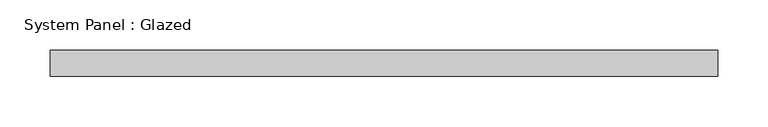
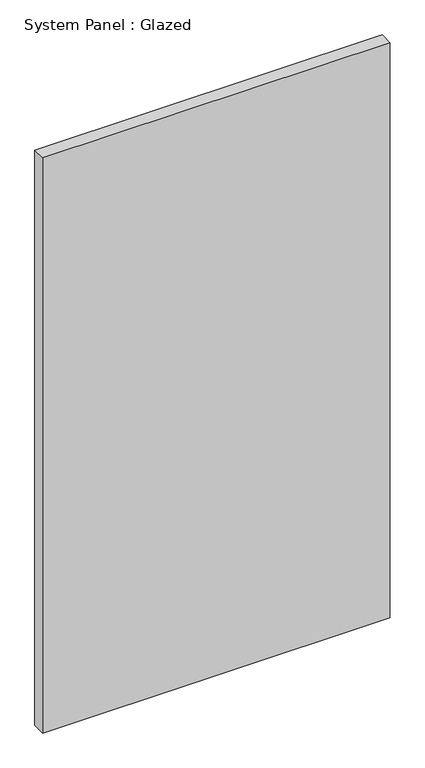
"""IFC4 building model written with IfcOpenShell, lengths in millimetres: plate geometry, System Panel : Glazed."""

from ifc_helpers import new_model, si_unit, origin, origin_with_axes, place, context, project, spatial, polyline, outline, extrude, source, transform, mapped, element, save


def system_panel_glazed_73c284ea(model_context):
    return source(origin(), model_context, "Body", "SweptSolid", [
        extrude(outline(polyline([(330.2, 19.05), (-330.2, 19.05), (-330.2, 44.45), (330.2, 44.45), (330.2, 19.05)])), origin_with_axes(), (0.0, 0.0, 1.0), 1155.7),
    ])


if __name__ == "__main__":
    model = new_model("IFC4")
    model_context = context("Model", 3, world=origin())
    ifc_project = project(units=[si_unit("LENGTHUNIT", "METRE", prefix="MILLI")], contexts=[model_context])
    site = spatial("IfcSite", under=ifc_project)
    building = spatial("IfcBuilding", under=site)
    placement = place(None, origin())
    system_panel_glazed_shape = system_panel_glazed_73c284ea(model_context)
    element("IfcPlate", 1, ObjectType="System Panel : Glazed", at=placement, inside=building, context=model_context, shape_type="MappedRepresentation", body=[
        mapped(system_panel_glazed_shape, transform((0.0, 0.0, 0.0), x_axis=(1.0, 0.0, 0.0), y_axis=(0.0, 1.0, 0.0), z_axis=(0.0, 0.0, 1.0))),
    ])
    save(model, "model.ifc")

# Revit data of these elements
# Type "System Panel : Glazed"
#   Construction Type Id = "GSP4R"
#   Analytic Construction = "1/8 in Pilkington single glazing"
#   Visual Light Transmittance = 0.9
#   Solar Heat Gain Coefficient = 0.86
#   Heat Transfer Coefficient (U) = 1.18115 BTU/(h·ft²·°F)
# Element 1 (IfcPlate, "System Panel : Glazed")
#   Materials on its faces: "Glass"
# Materials
#   "Glass": class "Glass", colour RGB 0 128 192, transparency 0.75, Description = "Soda Lime Glass", Cost = 0
